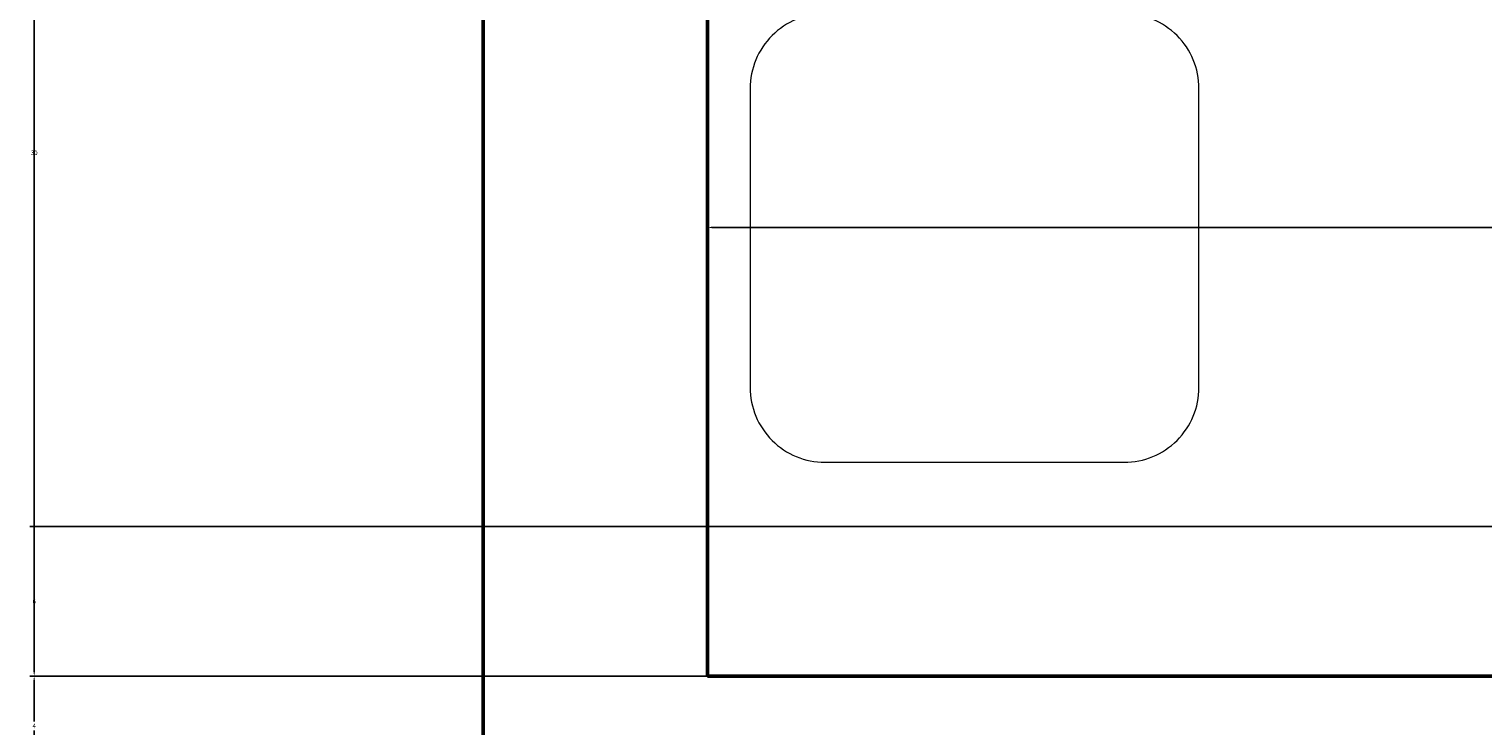
# Model space of a CAD drawing. Units: inches. Extents: x 2621 to 2849, y 2066 to 2463.
# Tile 13 of 28: x 2621 to 2679, y 2317 to 2345. Entities that reach past the tile are written whole.
import ezdxf

# ---------------------------------------------------------------- set-up
doc = ezdxf.new("R2010")
doc.units = ezdxf.units.IN
for name, color, linetype, lineweight in [('A-ANNO-DIMS', 2, 'Continuous', 18), ('A-FURN', 8, 'Continuous', 18), ('A-WALL', 7, 'Continuous', 50)]:
    doc.layers.add(name, color=color, linetype=linetype, lineweight=lineweight)
doc.styles.get("Standard").update_dxf_attribs({"font": 'arial.ttf'})
doc.dimstyles.get("Standard").update_dxf_attribs({"dimtxt": 0.18, "dimasz": 0.18, "dimexe": 0.18, "dimexo": 0.0625, "dimgap": 0.09, "dimtad": 0, "dimtih": 1, "dimtoh": 1, "dimdec": 4, "dimzin": 0, "dimdsep": 46, "dimtxsty": 'Standard', "dimcen": 0.09, "dimadec": 0, "dimazin": 0, "dimtfac": 1, "dimtdec": 4, "dimtofl": 0, "dimtmove": 0, "dimatfit": 3, "dimfxl": 1, "dimtolj": 1, "dimtzin": 0, "dimarcsym": 0})

# ---------------------------------------------------------------- blocks, each defined once
blk = doc.blocks.new('*D45')
at = {"layer": 'A-ANNO-DIMS', "color": 0, "lineweight": -2, "transparency": 16777216}
for p, q in [((2647.87, 2319.437), (2647.87, 2337.558)), ((2763.87, 2319.437), (2763.87, 2337.558)), ((2648.05, 2337.378), (2705.59, 2337.378)), ((2763.69, 2337.378), (2706.15, 2337.378))]:
    blk.add_line(p, q, dxfattribs=at)
at = {"layer": 'A-ANNO-DIMS', "color": 0, "transparency": 16777216}
for points in [[(2648.05, 2337.408), (2648.05, 2337.348), (2647.87, 2337.378)], [(2763.69, 2337.408), (2763.69, 2337.348), (2763.87, 2337.378)]]:
    blk.add_solid(points, dxfattribs=at)
at = {"layer": 'Defpoints', "color": 0, "transparency": 16777216}
for p in [(2763.87, 2337.378), (2647.87, 2319.375), (2763.87, 2319.375)]:
    blk.add_point(p, dxfattribs=at)
at = {"layer": 'A-ANNO-DIMS', "color": 0, "transparency": 16777216, "insert": (2705.87, 2337.378), "char_height": 0.18, "attachment_point": 5}
blk.add_mtext('\\A1;116', dxfattribs=at)
blk = doc.blocks.new('*D46')
at = {"layer": 'A-ANNO-DIMS', "color": 0, "lineweight": -2, "transparency": 16777216}
for p, q in [((2647.808, 2435.375), (2620.687, 2435.375)), ((2620.867, 2435.195), (2620.867, 2377.556)), ((2620.867, 2319.555), (2620.867, 2377.193)), ((2647.808, 2319.375), (2620.687, 2319.375))]:
    blk.add_line(p, q, dxfattribs=at)
at = {"layer": 'A-ANNO-DIMS', "color": 0, "transparency": 16777216}
for points in [[(2620.837, 2435.195), (2620.897, 2435.195), (2620.867, 2435.375)], [(2620.837, 2319.555), (2620.897, 2319.555), (2620.867, 2319.375)]]:
    blk.add_solid(points, dxfattribs=at)
at = {"layer": 'Defpoints', "color": 0, "transparency": 16777216}
for p in [(2620.867, 2435.375), (2647.87, 2435.375), (2647.87, 2319.375)]:
    blk.add_point(p, dxfattribs=at)
at = {"layer": 'A-ANNO-DIMS', "color": 0, "transparency": 16777216, "insert": (2620.867, 2377.375), "char_height": 0.18, "attachment_point": 5}
blk.add_mtext('\\A1;116', dxfattribs=at)
blk = doc.blocks.new('*D49')
at = {"layer": 'A-ANNO-DIMS', "color": 0, "lineweight": -2, "transparency": 16777216}
for p, q in [((2647.807599, 2319.374587), (2620.686599, 2319.374587)), ((2620.866599, 2319.194587), (2620.866599, 2317.554587)), ((2620.866599, 2315.554587), (2620.866599, 2317.194587)), ((2647.807599, 2315.374587), (2620.686599, 2315.374587))]:
    blk.add_line(p, q, dxfattribs=at)
at = {"layer": 'A-ANNO-DIMS', "color": 0, "transparency": 16777216}
for points in [[(2620.836599, 2319.194587), (2620.896599, 2319.194587), (2620.866599, 2319.374587)], [(2620.836599, 2315.554587), (2620.896599, 2315.554587), (2620.866599, 2315.374587)]]:
    blk.add_solid(points, dxfattribs=at)
at = {"layer": 'Defpoints', "color": 0, "transparency": 16777216}
for p in [(2647.870099, 2319.374587), (2620.866599, 2315.374587), (2647.870099, 2315.374587)]:
    blk.add_point(p, dxfattribs=at)
at = {"layer": 'A-ANNO-DIMS', "color": 0, "transparency": 16777216, "insert": (2620.866599, 2317.374587), "char_height": 0.18, "attachment_point": 5}
blk.add_mtext('\\A1;4', dxfattribs=at)
blk = doc.blocks.new('*D50')
at = {"layer": 'A-ANNO-DIMS', "color": 0, "lineweight": -2, "transparency": 16777216}
for p, q in [((2763.808, 2355.375), (2620.687, 2355.375)), ((2620.867, 2355.195), (2620.867, 2340.557)), ((2620.867, 2325.555), (2620.867, 2340.193)), ((2763.808, 2325.375), (2620.687, 2325.375))]:
    blk.add_line(p, q, dxfattribs=at)
at = {"layer": 'A-ANNO-DIMS', "color": 0, "transparency": 16777216}
for points in [[(2620.837, 2355.195), (2620.897, 2355.195), (2620.867, 2355.375)], [(2620.837, 2325.555), (2620.897, 2325.555), (2620.867, 2325.375)]]:
    blk.add_solid(points, dxfattribs=at)
at = {"layer": 'Defpoints', "color": 0, "transparency": 16777216}
for p in [(2620.867, 2355.375), (2763.87, 2355.375), (2763.87, 2325.375)]:
    blk.add_point(p, dxfattribs=at)
at = {"layer": 'A-ANNO-DIMS', "color": 0, "transparency": 16777216, "insert": (2620.867, 2340.375), "char_height": 0.18, "attachment_point": 5}
blk.add_mtext('\\A1;30', dxfattribs=at)
blk = doc.blocks.new('*D51')
at = {"layer": 'A-ANNO-DIMS', "color": 0, "lineweight": -2, "transparency": 16777216}
for p, q in [((2763.808, 2325.375), (2620.687, 2325.375)), ((2620.867, 2325.195), (2620.867, 2322.556)), ((2620.867, 2319.555), (2620.867, 2322.193)), ((2763.808, 2319.375), (2620.687, 2319.375))]:
    blk.add_line(p, q, dxfattribs=at)
at = {"layer": 'A-ANNO-DIMS', "color": 0, "transparency": 16777216}
for points in [[(2620.837, 2325.195), (2620.897, 2325.195), (2620.867, 2325.375)], [(2620.837, 2319.555), (2620.897, 2319.555), (2620.867, 2319.375)]]:
    blk.add_solid(points, dxfattribs=at)
at = {"layer": 'Defpoints', "color": 0, "transparency": 16777216}
for p in [(2620.867, 2325.375), (2763.87, 2325.375), (2763.87, 2319.375)]:
    blk.add_point(p, dxfattribs=at)
at = {"layer": 'A-ANNO-DIMS', "color": 0, "transparency": 16777216, "insert": (2620.867, 2322.375), "char_height": 0.18, "attachment_point": 5}
blk.add_mtext('\\A1;6', dxfattribs=at)

msp = doc.modelspace()

# ---------------------------------------------------------------- linework, layer by layer
at = {"layer": 'A-FURN'}
msp.add_lwpolyline([(2652.5811, 2327.9537), (2664.5811, 2327.9537, 0.4142136), (2667.5811, 2330.9537), (2667.5811, 2342.9537, 0.4142136), (2664.5811, 2345.9537), (2652.5811, 2345.9537, 0.4142136), (2649.5811, 2342.9537), (2649.5811, 2330.9537, 0.4142136)], format="xyb", close=True, dxfattribs=at)
at = {"layer": 'A-WALL'}
for q in [(2647.8701, 2435.3746), (2763.8701, 2319.3746)]:
    msp.add_line((2647.8701, 2319.3746), q, dxfattribs=at)
msp.add_lwpolyline([(2761.8701, 2084.3746), (2638.8701, 2084.3746), (2638.8701, 2444.3746), (2830.8701, 2444.3746), (2830.8701, 2084.3746), (2797.8701, 2084.3746)], dxfattribs=at)

# ---------------------------------------------------------------- dimensions: what is measured, and where the dimension line sits
at = {"layer": 'A-ANNO-DIMS'}
for base, p1, p2, picture, middle in [((2620.8666, 2435.3746), (2647.8701, 2319.3746), (2647.8701, 2435.3746), '*D46', (2620.8666, 2377.3746)), ((2620.8666, 2355.3746), (2763.8701, 2325.3746), (2763.8701, 2355.3746), '*D50', (2620.8666, 2340.3746)), ((2620.8666, 2325.3746), (2763.8701, 2319.3746), (2763.8701, 2325.3746), '*D51', (2620.8666, 2322.3746)), ((2620.8666, 2315.3746), (2647.8701, 2319.3746), (2647.8701, 2315.3746), '*D49', (2620.8666, 2317.3746))]:
    dim = msp.add_linear_dim(base=base, p1=p1, p2=p2, angle=90, dimstyle='Standard', override={"dimdec": 0, "dimlfac": 1, "dimrnd": 0, "dimzin": 0, "dimdsep": 46, "dimlunit": 2}, dxfattribs=at)
    dim.commit()
    dim.dimension.update_dxf_attribs({"geometry": picture, "text_midpoint": middle})
dim = msp.add_linear_dim(base=(2763.8701, 2337.3781), p1=(2647.8701, 2319.3746), p2=(2763.8701, 2319.3746), dimstyle='Standard', override={"dimdec": 0, "dimlfac": 1, "dimrnd": 0, "dimzin": 0, "dimdsep": 46, "dimlunit": 2}, dxfattribs=at)
dim.commit()
dim.dimension.update_dxf_attribs({"geometry": '*D45', "text_midpoint": (2705.8701, 2337.3781)})

doc.saveas('drawing.dxf')
